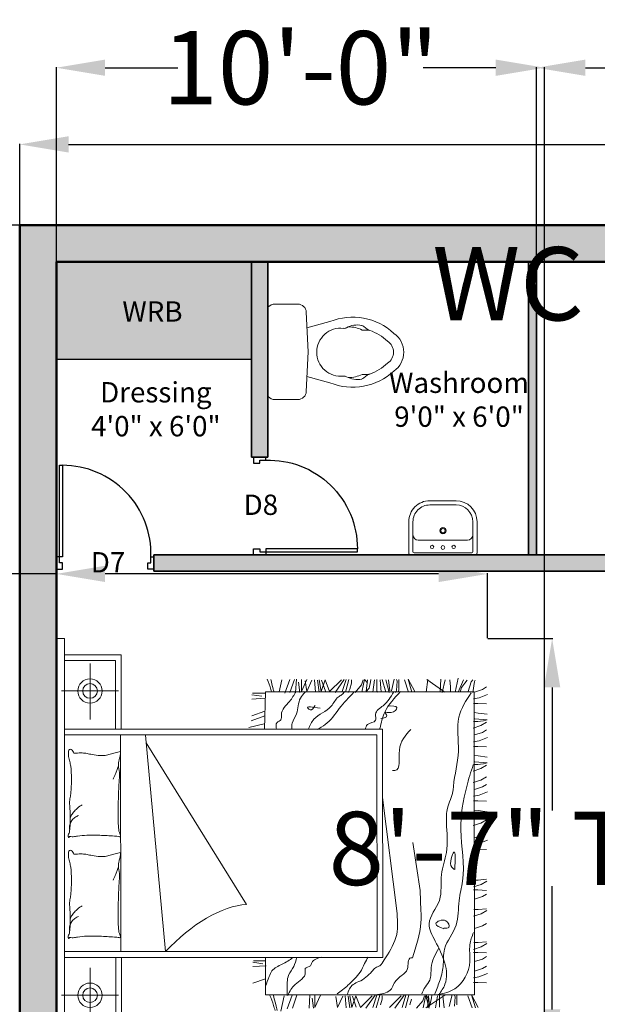
# Model space of a CAD drawing. Units: inches. Extents: x 2796 to 3603, y 978 to 1787.
# Tile 12 of 15: x 3070 to 3212, y 1545 to 1787. Entities that reach past the tile are written whole.
import ezdxf

# ---------------------------------------------------------------- set-up
doc = ezdxf.new("R2010")
doc.units = ezdxf.units.IN
for name, color, linetype, lineweight in [('A-ANNO-DIMS', 7, 'Continuous', 18), ('A-ANNO-TEXT', 7, 'Continuous', 18), ('A-AREA-IDEN', 7, 'Continuous', 18), ('A-DOOR', 6, 'Continuous', 25), ('A-FLOR-CASE', 2, 'Continuous', 25), ('A-FLOR-CASE-PATT', 2, 'Continuous', 13), ('A-FLOR-FIXT', 8, 'Continuous', 18), ('A-WALL-EXTR-PATT', 1, 'Continuous', 13), ('A-WALL-INTR-PATT', 5, 'Continuous', 13), ('Furniture', 2, 'Continuous', 18), ('Inner Wall', 5, 'Continuous', 35), ('Outer Wall', 1, 'Continuous', 50)]:
    doc.layers.add(name, color=color, linetype=linetype, lineweight=lineweight)
doc.styles.get("Standard").update_dxf_attribs({"font": 'arial.ttf'})
doc.dimstyles.get("Standard").update_dxf_attribs({"dimtxt": 18, "dimasz": 12, "dimexe": 0.18, "dimexo": 0.0625, "dimgap": 0.09, "dimtad": 0, "dimtih": 1, "dimtoh": 1, "dimdec": 0, "dimzin": 0, "dimdsep": 46, "dimlunit": 3, "dimtxsty": 'Standard', "dimcen": 0.09, "dimadec": 0, "dimazin": 0, "dimtfac": 1, "dimtdec": 0, "dimtofl": 0, "dimtmove": 0, "dimatfit": 3, "dimfxl": 1, "dimtolj": 1, "dimtzin": 0, "dimarcsym": 0})

# ---------------------------------------------------------------- blocks, each defined once
blk = doc.blocks.new('A$C1308471B')
at = {"ltscale": 20}
for p, q in [((0, 0.4607), (0, 0.0186)), ((0.0354, 0.4793), (0.1495, 0.4793)), ((0.2013, 0.2397), (0.1923, 0.4384)), ((0.1957, 0.3639), (0.3109, 0.3953)), ((0.5021, 0.3528), (0.4724, 0.3528)), ((0.4982, 0.3575), (0.4822, 0.3709)), ((0.2013, 0.2397), (0.1923, 0.0409)), ((0.1959, 0.1193), (0.3109, 0.0879)), ((0.5021, 0.1304), (0.4724, 0.1304)), ((0.4982, 0.1257), (0.4822, 0.1123)), ((0.0354, 0), (0.1495, 0))]:
    blk.add_line(p, q, dxfattribs=at)
for centre, radius, start, end in [((0.006, 0.4607), 0.006, 136.5269, 180), ((0.0354, 0.4328), 0.0465, 90, 136.5269), ((0.1495, 0.4365), 0.0429, 2.5755, 90), ((0.4248, 0.1104), 0.3068, 47.4135, 111.7924), ((0.3654, 0.2416), 0.1206, 83.3523, 180), ((0.3823, 0.3868), 0.0255, 263.3523, 298.5742), ((0.4494, 0.2636), 0.1148, 79.3968, 118.5742), ((0.405, 0.2159), 0.153, 63.502, 90.4522), ((0.4658, 0.3513), 0.0255, 50, 79.3968), ((0.5146, 0.377), 0.0255, 230, 251.3881), ((0.5021, 0.3273), 0.0255, 70.3751, 90), ((0.4248, 0.1104), 0.2558, 46.612, 70.3751), ((0.5654, 0.2416), 0.116, 0, 54.7115), ((0.5654, 0.2416), 0.065, 0, 57.2974), ((0.3654, 0.2416), 0.1206, 180, 276.6477), ((0.5654, 0.2416), 0.065, 302.7026, 0), ((0.5654, 0.2416), 0.116, 305.2885, 0), ((0.4248, 0.3728), 0.2558, 289.6249, 313.388), ((0.4248, 0.3728), 0.3068, 248.2076, 312.5865), ((0.3823, 0.0964), 0.0255, 61.4258, 96.6477), ((0.4494, 0.2196), 0.1148, 241.4258, 280.6032), ((0.405, 0.2673), 0.153, 269.5478, 296.498), ((0.4658, 0.1319), 0.0255, 280.6032, 310), ((0.5146, 0.1062), 0.0255, 108.6119, 130), ((0.5021, 0.1559), 0.0255, 270, 289.6249), ((0.006, 0.0186), 0.006, 180, 223.4731), ((0.0354, 0.0465), 0.0465, 223.4731, 270), ((0.1495, 0.0429), 0.0429, 270, 357.4245)]:
    blk.add_arc(centre, radius, start, end, dxfattribs=at)
blk = doc.blocks.new('A$C57EA129C')
for p, q in [((0, 0.4428), (0, 0.1782)), ((0.016, 0.4589), (0.5631, 0.4589)), ((0.0356, 0.4321), (0.0356, 0.2896)), ((0.0445, 0.441), (0.5346, 0.441)), ((0.5435, 0.4321), (0.5435, 0.2896)), ((0.5791, 0.4428), (0.5791, 0.1782)), ((0.0802, 0.3341), (0.499, 0.3341)), ((0.0356, 0.2896), (0.0356, 0.1782)), ((0.5435, 0.2896), (0.5435, 0.1782)), ((0.1782, 0.0356), (0.4009, 0.0356)), ((0.1782, 0), (0.4009, 0))]:
    blk.add_line(p, q)
for centre, radius in [((0.1982, 0.392), 0.0143), ((0.2896, 0.3965), 0.0156), ((0.3809, 0.392), 0.0143), ((0.2896, 0.2545), 0.0267), ((0.2896, 0.2545), 0.0178)]:
    blk.add_circle(centre, radius)
for centre, radius, start, end in [((0.016, 0.4428), 0.016, 90, 180), ((0.0445, 0.4321), 0.00891, 90, 180), ((0.5346, 0.4321), 0.00891, 0, 90), ((0.5631, 0.4428), 0.016, 0, 90), ((0.0802, 0.2896), 0.0445, 90, 180), ((0.499, 0.2896), 0.0445, 0, 90), ((0.1782, 0.1782), 0.1782, 180, 270), ((0.1782, 0.1782), 0.1426, 180, 270), ((0.4009, 0.1782), 0.1782, 270, 0), ((0.4009, 0.1782), 0.1426, 270, 0)]:
    blk.add_arc(centre, radius, start, end)
blk = doc.blocks.new('A$C2B723114')
for p, q in [((0, 2.9047), (2.8274, 2.9047)), ((0, 2.8487), (0, 2.9047)), ((0.4243, 2.8697), (0.4243, 2.4855)), ((2.4742, 2.8697), (2.4742, 2.4855)), ((2.8274, 2.9047), (2.8274, 2.8487)), ((2.8274, 2.8487), (0, 2.8487)), ((0.1012, 2.4649), (0.1012, 2.849)), ((0.1396, 2.5033), (0.1396, 2.849)), ((0.6794, 0.7051), (0.6794, 2.8509)), ((0.7187, 0.7435), (0.7187, 2.8509)), ((2.1776, 2.8509), (2.1776, 0.7454)), ((2.216, 2.8509), (2.216, 0.707)), ((2.6798, 2.5052), (2.6798, 2.8509)), ((2.7182, 2.4668), (2.7182, 2.8509)), ((0.6087, 2.6776), (0.295, 2.6776)), ((2.6586, 2.6776), (2.2821, 2.6776)), ((1.3789, 2.4999), (1.3598, 2.5761)), ((2.0593, 2.4999), (2.0402, 2.5761)), ((0.6794, 2.4649), (0.1012, 2.4649)), ((0.6766, 2.5033), (0.1396, 2.5033)), ((0.7191, 2.47), (2.1778, 2.4719)), ((1.3858, 2.4723), (1.3789, 2.4999)), ((2.0662, 2.4723), (2.0593, 2.4999)), ((2.2188, 2.5052), (2.6798, 2.5052)), ((2.2188, 2.4668), (2.7182, 2.4668)), ((2.1771, 2.3036), (0.718, 2.1685)), ((1.0365, 1.6233), (2.1246, 2.2989)), ((2.2287, 1.6076), (2.2523, 1.5035)), ((2.2726, 1.593), (2.3061, 1.5007)), ((0.5047, 1.5819), (0.5353, 1.4945)), ((0.6174, 1.5819), (0.6232, 1.4916)), ((0.6467, 1.5819), (0.6369, 1.5137)), ((0.6571, 1.4945), (0.6571, 1.5765)), ((2.3067, 1.5881), (2.3373, 1.5007)), ((2.4194, 1.5881), (2.4251, 1.4979)), ((2.4487, 1.5881), (2.4389, 1.5199)), ((2.4591, 1.5007), (2.4591, 1.5828)), ((0.4269, 0.0884), (0.4269, 1.4945)), ((0.4269, 1.4945), (0.6794, 1.4945)), ((2.4685, 1.4964), (2.216, 1.5022)), ((2.4685, 1.4964), (2.4685, 0.0903)), ((2.4685, 1.4044), (2.5491, 1.3861)), ((0.3172, 1.3923), (0.4213, 1.3687)), ((0.3318, 1.3485), (0.4241, 1.3149)), ((2.4596, 1.3659), (2.552, 1.3324)), ((2.4645, 1.3318), (2.552, 1.3012)), ((0.3367, 1.3143), (0.4241, 1.2838)), ((2.4645, 1.2928), (2.5548, 1.2871)), ((2.4645, 1.2635), (2.5328, 1.2733)), ((0.3367, 1.2016), (0.427, 1.1959)), ((2.4699, 1.2531), (2.552, 1.2163)), ((2.552, 1.2531), (2.4699, 1.2531)), ((2.5435, 1.2276), (2.4699, 1.2163)), ((2.4699, 1.2163), (2.5463, 1.1823)), ((0.3367, 1.1724), (0.405, 1.1821)), ((0.4241, 1.162), (0.3421, 1.162)), ((0.3421, 1.162), (0.4241, 1.1252)), ((2.5491, 1.1654), (2.467, 1.1597)), ((2.5463, 1.1455), (2.467, 1.1342)), ((2.5491, 1.1342), (2.4699, 1.1201)), ((2.4699, 1.1201), (2.5491, 1.0946)), ((2.5491, 1.0946), (2.4699, 1.0635)), ((2.4699, 1.0635), (2.5491, 0.9842)), ((2.5463, 1.1172), (2.4727, 1.0918)), ((0.4157, 1.0206), (0.3421, 1.0093)), ((0.3421, 1.0093), (0.4185, 0.9754)), ((2.4642, 1.0267), (2.552, 0.9644)), ((0.4213, 0.9584), (0.3392, 0.9527)), ((0.4185, 0.9386), (0.3392, 0.9272)), ((2.4642, 0.9389), (2.4869, 0.9276)), ((2.467, 0.9559), (2.552, 0.9333)), ((2.4699, 0.9785), (2.552, 0.9531)), ((0.4213, 0.9272), (0.3421, 0.9131)), ((0.3421, 0.9131), (0.4213, 0.8876)), ((0.4213, 0.8876), (0.3421, 0.8565)), ((0.4185, 0.9103), (0.3449, 0.8848)), ((2.4642, 0.8908), (2.5152, 0.8483)), ((2.4869, 0.9276), (2.5265, 0.9163)), ((2.5265, 0.9163), (2.5491, 0.9163)), ((0.3364, 0.8197), (0.4241, 0.7574)), ((0.3421, 0.8565), (0.4213, 0.7772)), ((2.467, 0.8455), (2.5208, 0.8342)), ((2.4699, 0.8172), (2.4925, 0.7974)), ((2.5491, 0.8087), (2.4699, 0.8172)), ((2.4925, 0.7974), (2.535, 0.7889)), ((2.5152, 0.8483), (2.5491, 0.837)), ((2.5208, 0.8342), (2.552, 0.8285)), ((2.552, 0.8285), (2.5293, 0.8087)), ((0.3392, 0.7489), (0.4241, 0.7263)), ((0.3421, 0.7716), (0.4241, 0.7461)), ((2.1776, 0.7454), (0.7187, 0.7435)), ((2.5491, 0.7606), (2.467, 0.7719)), ((2.4727, 0.7464), (2.467, 0.7408)), ((2.552, 0.7464), (2.4727, 0.7464)), ((2.535, 0.7889), (2.552, 0.7861)), ((0.359, 0.7206), (0.3987, 0.7093)), ((0.3987, 0.7093), (0.4213, 0.7093)), ((2.216, 0.707), (0.6794, 0.7051)), ((0.9938, 0.6115), (1.7555, 0.7064)), ((2.5491, 0.6842), (2.4642, 0.6615)), ((2.467, 0.7153), (2.5491, 0.7238)), ((2.552, 0.7096), (2.467, 0.6842)), ((2.5491, 0.6672), (2.4755, 0.6587)), ((0.3364, 0.6233), (0.4241, 0.561)), ((0.3421, 0.6601), (0.4213, 0.5808)), ((2.4642, 0.6191), (2.4784, 0.6134)), ((2.467, 0.5993), (2.4869, 0.5964)), ((2.4755, 0.6474), (2.5548, 0.6276)), ((2.4784, 0.6134), (2.5406, 0.6077)), ((2.5406, 0.6077), (2.552, 0.6134)), ((0.3392, 0.5525), (0.4241, 0.5299)), ((0.3421, 0.5752), (0.4241, 0.5497)), ((2.467, 0.5313), (2.5491, 0.5596)), ((2.467, 0.5087), (2.5548, 0.5342)), ((2.5548, 0.5342), (2.4699, 0.4889)), ((2.4869, 0.5964), (2.552, 0.5964)), ((0.3364, 0.4785), (0.3874, 0.436)), ((0.359, 0.5242), (0.3987, 0.5129)), ((1.4523, 0.5021), (1.1305, 0.4537)), ((0.4213, 0.415), (0.3364, 0.3923)), ((0.3392, 0.4332), (0.393, 0.4219)), ((0.4241, 0.2868), (0.3392, 0.415)), ((0.3421, 0.4049), (0.3647, 0.3851)), ((0.4213, 0.3964), (0.3421, 0.4049)), ((0.3874, 0.436), (0.4213, 0.4247)), ((0.393, 0.4219), (0.4241, 0.4162)), ((0.4241, 0.4162), (0.4015, 0.3964)), ((1.1305, 0.4537), (0.9938, 0.448)), ((2.467, 0.4133), (2.552, 0.4019)), ((2.467, 0.2879), (2.552, 0.4076)), ((0.4213, 0.3377), (0.3392, 0.3491)), ((0.4213, 0.398), (0.3477, 0.3895)), ((0.3647, 0.3851), (0.4072, 0.3766)), ((0.4072, 0.3766), (0.4241, 0.3738)), ((0.3392, 0.2925), (0.4213, 0.3009)), ((0.4241, 0.3236), (0.3449, 0.3236)), ((2.4642, 0.3049), (2.5491, 0.2851)), ((2.467, 0.319), (2.5548, 0.3134)), ((0.3477, 0.2571), (0.427, 0.2373)), ((0.3506, 0.2231), (0.4128, 0.2175)), ((0.359, 0.2061), (0.4241, 0.2061)), ((0.4128, 0.2175), (0.4241, 0.2231)), ((2.467, 0.2179), (2.5605, 0.1981)), ((2.4699, 0.2491), (2.501, 0.2491)), ((2.501, 0.2491), (2.5491, 0.2547)), ((2.467, 0.1981), (2.5491, 0.1613)), ((2.467, 0.184), (2.4982, 0.1755)), ((2.4982, 0.1755), (2.5463, 0.1359)), ((0.3392, 0.1042), (0.4213, 0.1325)), ((0.3392, 0.0815), (0.427, 0.107)), ((0.427, 0.107), (0.3421, 0.0617)), ((2.4685, 0.0903), (0.4269, 0.0884)), ((0.5106, 0.094), (0.5106, 0.0657)), ((0.5417, 0.094), (0.5474, 0.0572)), ((0.587, 0.0884), (0.604, 0.0346)), ((0.6512, 0.0884), (0.6682, 0.0346)), ((0.713, 0.094), (0.713, 0.0657)), ((0.7334, 0.0943), (0.7503, 0.0434)), ((0.7786, 0.0915), (0.7786, 0.0632)), ((0.8739, 0.0884), (0.8908, 0.0346)), ((0.956, 0.0943), (0.973, 0.0434)), ((1.0013, 0.0915), (1.0013, 0.0632)), ((1.072, 0.0884), (1.089, 0.0346)), ((1.1338, 0.094), (1.1338, 0.0657)), ((1.1542, 0.0943), (1.1712, 0.0434)), ((1.1995, 0.0915), (1.1995, 0.0632)), ((1.4088, 0.094), (1.4088, 0.0657)), ((1.44, 0.094), (1.4456, 0.0572)), ((1.4853, 0.0884), (1.5023, 0.0346)), ((1.5674, 0.0962), (1.5844, 0.0453)), ((1.6127, 0.0934), (1.6127, 0.0651)), ((1.6297, 0.0849), (1.624, 0.0028)), ((1.6721, 0.0877), (1.6693, 0.0623)), ((1.7344, 0.0934), (1.7344, 0.0651)), ((1.7655, 0.0934), (1.7712, 0.0566)), ((1.8108, 0.0877), (1.8278, 0.034)), ((1.8568, 0.0962), (1.8738, 0.0453)), ((1.9342, 0.0962), (1.9512, 0.0453)), ((1.9795, 0.0934), (1.9795, 0.0651)), ((1.9965, 0.0849), (1.9908, 0.0028)), ((2.039, 0.0877), (2.0361, 0.0623)), ((2.1012, 0.0934), (2.1012, 0.0651)), ((2.1324, 0.0934), (2.138, 0.0566)), ((2.1777, 0.0877), (2.1946, 0.034)), ((2.2236, 0.0962), (2.2406, 0.0453)), ((2.2689, 0.0934), (2.2689, 0.0651)), ((2.2859, 0.0849), (2.2802, 0.0028)), ((2.3284, 0.0877), (2.3255, 0.0623)), ((2.3906, 0.0934), (2.3906, 0.0651)), ((2.4218, 0.0934), (2.4274, 0.0566)), ((2.4642, 0.0991), (2.5378, 0.0877)), ((2.467, 0.0877), (2.484, 0.034)), ((2.4699, 0.1302), (2.535, 0.1104)), ((2.535, 0.1104), (2.5491, 0.0991)), ((2.5378, 0.0877), (2.5463, 0.0821)), ((0.5106, 0.0657), (0.5077, 0.0063)), ((0.5474, 0.0572), (0.57, 0.0006)), ((0.604, 0.0346), (0.621, 0.0063)), ((0.6682, 0.0346), (0.6851, 0.0063)), ((0.713, 0.0657), (0.7101, 0.0063)), ((0.7503, 0.0434), (0.773, 0.0037)), ((0.7786, 0.0632), (0.7843, 0.0066)), ((0.8908, 0.0346), (0.9078, 0.0063)), ((0.973, 0.0434), (0.9957, 0.0037)), ((1.0013, 0.0632), (1.007, 0.0066)), ((1.089, 0.0346), (1.106, 0.0063)), ((1.1338, 0.0657), (1.131, 0.0063)), ((1.1712, 0.0434), (1.1939, 0.0037)), ((1.1995, 0.0632), (1.2052, 0.0066)), ((1.4088, 0.0657), (1.406, 0.0063)), ((1.4456, 0.0572), (1.4683, 0.0006)), ((1.5023, 0.0346), (1.5192, 0.0082)), ((1.5844, 0.0453), (1.607, 0.0057)), ((1.6127, 0.0651), (1.6184, 0.0085)), ((1.6693, 0.0623), (1.6608, 0.0028)), ((1.7344, 0.0651), (1.7316, 0.0057)), ((1.7712, 0.0566), (1.7938, 0)), ((1.8278, 0.034), (1.8448, 0.0057)), ((1.8738, 0.0453), (1.8964, 0.0057)), ((1.9512, 0.0453), (1.9739, 0.0057)), ((1.9795, 0.0651), (1.9852, 0.0085)), ((2.0361, 0.0623), (2.0276, 0.0028)), ((2.1012, 0.0651), (2.0984, 0.0057)), ((2.138, 0.0566), (2.1607, 0)), ((2.1946, 0.034), (2.2116, 0.0057)), ((2.2406, 0.0453), (2.2632, 0.0057)), ((2.2689, 0.0651), (2.2746, 0.0085)), ((2.3255, 0.0623), (2.317, 0.0028)), ((2.3906, 0.0651), (2.3878, 0.0057)), ((2.4274, 0.0566), (2.4501, 0)), ((2.484, 0.034), (2.501, 0.0057))]:
    blk.add_line(p, q)
for centre, radius in [((0.4243, 2.6776), 0.0821), ((0.4243, 2.6776), 0.0493), ((2.4742, 2.6776), 0.0821), ((2.4742, 2.6776), 0.0493)]:
    blk.add_circle(centre, radius)
for centre, radius, start, end in [((0.8078, 2.821), 0.00214, 160.43603, 281.89306), ((0.8088, 2.8207), 0.00315, 111.7883, 160.43603), ((0.8162, 2.8021), 0.0232, 94.30254, 111.7883), ((0.8091, 2.8151), 0.00394, 21.9904, 101.89306), ((0.8409, 2.7949), 0.0302, 158.57902, 188.13348), ((1.0356, 2.8227), 0.2268, 188.13348, 192.10946), ((0.7994, 2.8112), 0.0144, 338.57902, 21.9904), ((0.8165, 2.7987), 0.0266, 59.34875, 94.30254), ((0.8554, 2.8643), 0.0497, 239.34875, 264.74081), ((0.9202, 3.5684), 0.7568, 264.74081, 268.09211), ((0.8679, 2.7254), 0.0915, 74.06476, 94.21588), ((0.8679, 2.7254), 0.0915, 53.91364, 74.06476), ((0.9409, 4.189), 1.3777, 268.09211, 270.57574), ((0.8679, 2.7254), 0.0915, 36.17665, 53.91364), ((0.86, 2.6097), 0.2158, 62.76041, 69.13972), ((0.9466, 3.6164), 0.8051, 270.57574, 274.80185), ((0.9263, 2.7386), 0.0708, 51.61143, 62.76041), ((0.7461, 2.511), 0.3611, 46.18849, 51.61143), ((1.0364, 2.548), 0.2671, 87.46141, 94.80185), ((1.042, 2.6745), 0.1405, 79.81012, 87.46141), ((1.1532, 3.2931), 0.488, 259.81012, 263.9133), ((1.204, 3.7695), 0.9671, 263.9133, 270), ((1.204, 3.4318), 0.6294, 270, 277.54685), ((1.2573, 3.0292), 0.2233, 277.54685, 285.74398), ((1.3941, 2.5438), 0.281, 98.43719, 105.74398), ((1.3747, 2.6748), 0.1486, 90, 98.43719), ((1.3713, 2.8186), 0.0315, 274.40021, 333.41948), ((0.923, 2.7382), 0.4535, 0, 6.23236), ((1.3747, 2.74), 0.0833, 78.72762, 90), ((1.3886, 2.8099), 0.0121, 333.41948, 78.72762), ((1.4882, 2.821), 0.00214, 160.43603, 281.89306), ((1.4892, 2.8207), 0.00315, 111.7883, 160.43603), ((1.4966, 2.8021), 0.0232, 94.30254, 111.7883), ((1.4895, 2.8151), 0.00394, 21.9904, 101.89306), ((1.5213, 2.7949), 0.0302, 158.57902, 188.13348), ((1.716, 2.8227), 0.2268, 188.13348, 192.10946), ((1.4798, 2.8112), 0.0144, 338.57902, 21.9904), ((1.4969, 2.7987), 0.0266, 59.34875, 94.30254), ((1.5358, 2.8643), 0.0497, 239.34875, 264.74081), ((1.6006, 3.5684), 0.7568, 264.74081, 268.09211), ((1.5483, 2.7254), 0.0915, 74.06476, 94.21588), ((1.5483, 2.7254), 0.0915, 53.91364, 74.06476), ((1.6213, 4.189), 1.3777, 268.09211, 270.57574), ((1.5483, 2.7254), 0.0915, 36.17665, 53.91364), ((1.5404, 2.6097), 0.2158, 62.76041, 69.13972), ((1.627, 3.6164), 0.8051, 270.57574, 274.80185), ((1.6067, 2.7386), 0.0708, 51.61143, 62.76041), ((1.4265, 2.511), 0.3611, 46.18849, 51.61143), ((1.7168, 2.548), 0.2671, 87.46141, 94.80185), ((1.7224, 2.6745), 0.1405, 79.81012, 87.46141), ((1.8336, 3.2931), 0.488, 259.81012, 263.9133), ((1.8844, 3.7695), 0.9671, 263.9133, 270), ((1.8844, 3.4318), 0.6294, 270, 277.54685), ((1.9377, 3.0292), 0.2233, 277.54685, 285.74398), ((2.0745, 2.5438), 0.281, 98.43719, 105.74398), ((2.0551, 2.6748), 0.1486, 90, 98.43719), ((2.0517, 2.8186), 0.0315, 274.40021, 333.41948), ((1.6034, 2.7382), 0.4535, 0, 6.23236), ((2.0551, 2.74), 0.0833, 78.72762, 90), ((2.069, 2.8099), 0.0121, 333.41948, 78.72762), ((0.635, 2.7368), 0.1829, 7.6809, 12.10946), ((-0.0181, 2.6487), 0.8418, 3.36875, 7.6809), ((0.8679, 2.7254), 0.0915, 18.43965, 36.17665), ((0.8523, 2.6218), 0.2076, 39.03494, 46.18849), ((0.9783, 2.7239), 0.0455, 28.31676, 39.03494), ((0.8558, 2.6579), 0.1846, 23.00277, 28.31676), ((1.1884, 2.7382), 0.1881, 350.31563, 0), ((1.3154, 2.7368), 0.1829, 7.6809, 12.10946), ((0.6623, 2.6487), 0.8418, 3.36875, 7.6809), ((1.5483, 2.7254), 0.0915, 18.43965, 36.17665), ((1.5327, 2.6218), 0.2076, 39.03494, 46.18849), ((1.6587, 2.7239), 0.0455, 28.31676, 39.03494), ((1.5362, 2.6579), 0.1846, 23.00277, 28.31676), ((1.8688, 2.7382), 0.1881, 350.31563, 0), ((0.1976, 2.6614), 0.6258, 358.36691, 3.36875), ((1.6528, 2.6098), 0.2924, 167.80162, 171.99495), ((0.5722, 2.8434), 0.8132, 347.80162, 350.31563), ((0.878, 2.6614), 0.6258, 358.36691, 3.36875), ((2.3332, 2.6098), 0.2924, 167.80162, 171.99495), ((1.2526, 2.8434), 0.8132, 347.80162, 350.31563), ((-11.7321, 3.2823), 12.5718, 356.49514, 356.94504), ((-0.4351, 2.6794), 1.2587, 356.94504, 358.36691), ((1.9648, 2.5659), 0.6074, 171.99495, 177.33512), ((1.4204, 2.5912), 0.0624, 177.33512, 194.04519), ((-11.0517, 3.2823), 12.5718, 356.49514, 356.94504), ((0.2453, 2.6794), 1.2587, 356.94504, 358.36691), ((2.6452, 2.5659), 0.6074, 171.99495, 177.33512), ((2.1008, 2.5912), 0.0624, 177.33512, 194.04519), ((0.8298, 2.4774), 0.0178, 170.00164, 196.69777), ((0.5206, 2.5319), 0.2961, 350.00164, 356.49514), ((0.8139, 2.4726), 0.00122, 196.69777, 277.12039), ((0.8041, 2.5514), 0.0807, 277.12039, 286.22115), ((0.8068, 2.5419), 0.0707, 286.22115, 297.28412), ((0.8584, 2.4419), 0.0418, 102.86904, 117.28412), ((0.879, 2.3515), 0.1345, 93.57397, 102.86904), ((0.9376, 1.4146), 1.0732, 90.28654, 93.57397), ((0.9586, -2.7845), 5.2724, 89.02962, 90.28654), ((0.9954, -0.6123), 3.0999, 87.39037, 89.02962), ((1.0854, 1.364), 1.1216, 85.38242, 87.39037), ((1.28, 3.7729), 1.2952, 265.38242, 267.25094), ((1.4917, 3.1364), 0.681, 244.68893, 246.51559), ((1.228, 2.691), 0.2121, 267.25094, 281.55856), ((1.4917, 3.1364), 0.681, 246.51559, 248.34226), ((1.4917, 3.1364), 0.681, 248.34226, 250.57202), ((1.4917, 3.1364), 0.681, 250.57202, 252.80178), ((1.2975, 2.3514), 0.1345, 83.56595, 101.55856), ((1.3002, 2.3754), 0.1104, 72.61359, 83.56595), ((1.3965, 2.6828), 0.2118, 252.61359, 260.5159), ((1.4027, 2.7202), 0.2496, 260.5159, 265.91706), ((1.385, 2.4721), 0.000845, 265.91706, 14.04494), ((1.5102, 2.4774), 0.0178, 170.00164, 196.69777), ((1.201, 2.5319), 0.2961, 350.00164, 356.49514), ((1.4943, 2.4726), 0.00122, 196.69777, 277.12039), ((1.4845, 2.5514), 0.0807, 277.12039, 286.22115), ((1.4872, 2.5419), 0.0707, 286.22115, 297.28412), ((1.5388, 2.4419), 0.0418, 102.86904, 117.28412), ((1.5594, 2.3515), 0.1345, 93.57397, 102.86904), ((1.618, 1.4146), 1.0732, 90.28654, 93.57397), ((1.639, -2.7845), 5.2724, 89.02962, 90.28654), ((1.6758, -0.6123), 3.0999, 87.39037, 89.02962), ((1.7658, 1.364), 1.1216, 85.38242, 87.39037), ((1.9604, 3.7729), 1.2952, 265.38242, 267.25094), ((2.1721, 3.1364), 0.681, 244.68893, 246.51559), ((1.9084, 2.691), 0.2121, 267.25094, 281.55856), ((2.1721, 3.1364), 0.681, 246.51559, 248.34226), ((2.1721, 3.1364), 0.681, 248.34226, 250.57202), ((2.1721, 3.1364), 0.681, 250.57202, 252.80178), ((1.9779, 2.3514), 0.1345, 83.56595, 101.55856), ((1.9806, 2.3754), 0.1104, 72.61359, 83.56595), ((2.0769, 2.6828), 0.2118, 252.61359, 260.5159), ((2.0831, 2.7202), 0.2496, 260.5159, 265.91706), ((2.0654, 2.4721), 0.000845, 265.91706, 14.04494)]:
    blk.add_arc(centre, radius, start, end)
blk.add_ellipse((0.4962, 1.9132), major_axis=(0.4887, -0.4605), ratio=0.503305, start_param=0.491272, end_param=1.591113)
for points, knots in [([(0.427, 1.4678), (0.4036, 1.4582), (0.3693, 1.4441), (0.3335, 1.4344), (0.3221, 1.4313)], [0, 0, 0, 0, 98.452083, 144.639601, 144.639601, 144.639601, 144.639601]), ([(0.6768, 1.3104), (0.6615, 1.3339), (0.6315, 1.3797), (0.604, 1.4501), (0.5417, 1.4748), (0.5064, 1.4871), (0.4848, 1.4945)], [0, 0, 0, 0, 110.980521, 216.571322, 273.316778, 363.252298, 363.252298, 363.252298, 363.252298]), ([(2.5548, 1.4853), (2.5314, 1.4757), (2.5031, 1.4641), (2.4737, 1.4555), (2.4685, 1.454)], [0, 0, 0, 0, 98.452083, 119.481049, 119.481049, 119.481049, 119.481049]), ([(2.552, 1.4598), (2.5309, 1.4545), (2.5031, 1.4475), (2.4753, 1.4406), (2.4685, 1.4389)], [0, 0, 0, 0, 84.638756, 111.94623, 111.94623, 111.94623, 111.94623]), ([(0.4241, 1.4423), (0.4031, 1.437), (0.3691, 1.4284), (0.3351, 1.4199), (0.3221, 1.4167)], [0, 0, 0, 0, 84.638756, 136.955563, 136.955563, 136.955563, 136.955563]), ([(2.2145, 1.4211), (2.233, 1.4246), (2.2636, 1.4303), (2.2761, 1.3837), (2.3429, 1.3967), (2.3949, 1.3342), (2.4474, 1.3031), (2.4698, 1.2898)], [0, 0, 0, 0, 61.886907, 102.717887, 145.699352, 284.082577, 386.765171, 386.765171, 386.765171, 386.765171]), ([(0.6768, 1.286), (0.6567, 1.2911), (0.6145, 1.3017), (0.5543, 1.3533), (0.4816, 1.349), (0.4362, 1.3493), (0.4233, 1.3493)], [0, 0, 0, 0, 80.250278, 168.388677, 295.908361, 346.663112, 346.663112, 346.663112, 346.663112]), ([(0.4233, 1.3445), (0.4367, 1.3385), (0.464, 1.3264), (0.5129, 1.2848), (0.5456, 1.2161), (0.6131, 1.2349), (0.6142, 1.1913), (0.6642, 1.1806), (0.674, 1.144), (0.6817, 1.1154)], [0, 0, 0, 0, 56.745495, 115.23739, 254.956954, 286.678662, 337.828324, 366.201072, 468.500395, 468.500395, 468.500395, 468.500395]), ([(2.2145, 1.319), (2.2295, 1.319), (2.2678, 1.3192), (2.3288, 1.2705), (2.4143, 1.279), (2.4535, 1.2403), (2.4662, 1.2278)], [0, 0, 0, 0, 57.155505, 146.33427, 287.936209, 355.396728, 355.396728, 355.396728, 355.396728]), ([(2.2182, 1.2059), (2.2419, 1.1958), (2.3116, 1.1659), (2.342, 1.0552), (2.4266, 1.0223), (2.4474, 0.9811), (2.462, 0.9684), (2.4698, 0.9616)], [0, 0, 0, 0, 97.73655, 287.59661, 389.176293, 423.403759, 463.679181, 463.679181, 463.679181, 463.679181]), ([(2.3573, 1.127), (2.3656, 1.1759), (2.3758, 1.2352), (2.3371, 1.1853), (2.3602, 1.1713), (2.3768, 1.1612)], [0, 0, 0, 0, 107.853607, 130.728419, 189.220329, 189.220329, 189.220329, 189.220329]), ([(2.2145, 1.1476), (2.2246, 1.1286), (2.2575, 1.0666), (2.3612, 1.0009), (2.431, 0.9336), (2.4662, 0.8996)], [0, 0, 0, 0, 83.02987, 271.460712, 463.033803, 463.033803, 463.033803, 463.033803]), ([(0.6817, 0.8034), (0.6673, 0.8119), (0.6341, 0.8315), (0.5785, 0.8518), (0.5349, 0.8973), (0.4828, 0.9461), (0.4518, 0.9879), (0.4331, 1.013)], [0, 0, 0, 0, 65.318952, 150.437229, 226.833166, 307.58338, 429.454095, 429.454095, 429.454095, 429.454095]), ([(0.4282, 0.9448), (0.4547, 0.9353), (0.496, 0.9206), (0.5223, 0.8436), (0.5628, 0.7946), (0.6113, 0.7575), (0.6214, 0.7173), (0.6539, 0.7022), (0.672, 0.6897), (0.6768, 0.6864)], [0, 0, 0, 0, 102.299436, 159.044876, 303.717955, 348.579152, 391.138254, 454.581655, 477.456496, 477.456496, 477.456496, 477.456496]), ([(2.2145, 0.823), (2.227, 0.8201), (2.261, 0.8121), (2.261, 0.7401), (2.3352, 0.7659), (2.379, 0.6836), (2.4336, 0.6521), (2.4662, 0.6334)], [0, 0, 0, 0, 46.747668, 127.438174, 179.649794, 280.561838, 429.605131, 429.605131, 429.605131, 429.605131]), ([(0.4282, 0.74), (0.4347, 0.7029), (0.444, 0.6496), (0.5194, 0.6274), (0.555, 0.5807), (0.5975, 0.5243), (0.6789, 0.5415), (0.677, 0.5095), (0.6768, 0.5061)], [0, 0, 0, 0, 130.791737, 187.537266, 286.231946, 353.673191, 460.023761, 472.712403, 472.712403, 472.712403, 472.712403]), ([(0.6768, 0.6864), (0.7275, 0.655), (0.8251, 0.5944), (0.9391, 0.606), (0.9938, 0.6115)], [0, 0, 0, 0, 225.995823, 434.686543, 434.686543, 434.686543, 434.686543]), ([(2.2218, 0.7246), (2.2595, 0.716), (2.3548, 0.6945), (2.4265, 0.6268), (2.4698, 0.586)], [0, 0, 0, 0, 148.665024, 375.555892, 375.555892, 375.555892, 375.555892]), ([(2.3719, 0.6737), (2.3738, 0.6431), (2.3772, 0.5878), (2.3146, 0.6382), (2.3401, 0.7015), (2.2971, 0.6649), (2.2923, 0.6965), (2.289, 0.7176)], [0, 0, 0, 0, 83.446591, 150.887818, 201.642461, 230.015204, 286.760644, 286.760644, 286.760644, 286.760644]), ([(2.2145, 0.5167), (2.1764, 0.5522), (2.1051, 0.6184), (1.9357, 0.5803), (1.9385, 0.6342), (1.9388, 0.6395)], [0, 0, 0, 0, 208.073343, 389.01094, 409.01094, 409.01094, 409.01094, 409.01094]), ([(0.6768, 0.5061), (0.7554, 0.4794), (0.8591, 0.4442), (0.9675, 0.4473), (0.9938, 0.448)], [0, 0, 0, 0, 319.374611, 421.61723, 421.61723, 421.61723, 421.61723]), ([(0.4331, 0.4427), (0.4498, 0.4356), (0.4827, 0.4216), (0.5314, 0.3759), (0.632, 0.3884), (0.6996, 0.3513), (0.7423, 0.3278)], [0, 0, 0, 0, 70.931849, 139.556414, 248.154027, 434.709995, 434.709995, 434.709995, 434.709995]), ([(2.4625, 0.1088), (2.4095, 0.1438), (2.2904, 0.2226), (2.0623, 0.1771), (1.9006, 0.2246), (1.7699, 0.2337), (1.6941, 0.2766), (1.5528, 0.2786), (1.4005, 0.2587), (1.2324, 0.3267), (1.059, 0.2939), (0.9218, 0.426), (0.7359, 0.3204), (0.5586, 0.2391), (0.4502, 0.3116), (0.427, 0.3272)], [0, 0, 0, 0, 239.874704, 538.942419, 850.40885, 893.390315, 1047.998294, 1176.505142, 1437.500972, 1637.333004, 1864.324391, 2089.058767, 2248.736533, 2637.953392, 2744.252142, 2744.252142, 2744.252142, 2744.252142]), ([(1.9771, 0.0962), (1.9286, 0.1117), (1.7864, 0.157), (1.5223, 0.1992), (1.2611, 0.141), (1.0527, 0.2023), (0.8859, 0.1885), (0.76, 0.3042), (0.6211, 0.292), (0.5187, 0.3203), (0.4572, 0.3456), (0.4282, 0.3575)], [0, 0, 0, 0, 198.710624, 582.73994, 1031.873213, 1206.082894, 1423.278209, 1655.952104, 1808.744089, 1945.69963, 2068.229211, 2068.229211, 2068.229211, 2068.229211]), ([(0.8474, 0.0943), (0.82, 0.1047), (0.757, 0.1287), (0.6201, 0.1029), (0.4623, 0.1837), (0.4372, 0.2936), (0.4282, 0.3331)], [0, 0, 0, 0, 112.422038, 258.341957, 533.791494, 688.286079, 688.286079, 688.286079, 688.286079]), ([(0.8718, 0.2941), (0.8821, 0.3221), (0.9041, 0.3814), (0.9523, 0.2773), (0.8733, 0.2454), (0.8757, 0.2798), (0.8766, 0.2941)], [0, 0, 0, 0, 82.720021, 175.094899, 237.579423, 282.440623, 282.440623, 282.440623, 282.440623]), ([(1.2715, 0.221), (1.3344, 0.2172), (1.4529, 0.21), (1.2971, 0.2665), (1.2756, 0.2284), (1.2715, 0.221)], [0, 0, 0, 0, 150.888188, 283.977876, 315.699589, 315.699589, 315.699589, 315.699589])]:
    blk.add_open_spline(points, degree=3, knots=knots)
blk = doc.blocks.new('*D12')
at = {"layer": 'A-ANNO-DIMS', "color": 0, "lineweight": -2, "transparency": 16777216}
for p, q in [((3070.18, 1736.68), (3041.33, 1736.68)), ((3041.51, 1724.68), (3041.51, 1391.96)), ((3041.51, 1040.68), (3041.51, 1373.4)), ((3070.18, 1028.68), (3041.33, 1028.68))]:
    blk.add_line(p, q, dxfattribs=at)
at = {"layer": 'A-ANNO-DIMS', "color": 0, "transparency": 16777216}
for points in [[(3039.51, 1724.68), (3043.51, 1724.68), (3041.51, 1736.68)], [(3039.51, 1040.68), (3043.51, 1040.68), (3041.51, 1028.68)]]:
    blk.add_solid(points, dxfattribs=at)
at = {"layer": 'Defpoints', "color": 0, "transparency": 16777216}
for p in [(3041.51, 1736.68), (3070.25, 1736.68), (3070.25, 1028.68)]:
    blk.add_point(p, dxfattribs=at)
at = {"layer": 'A-ANNO-DIMS', "color": 0, "transparency": 16777216, "insert": (3041.51, 1382.68), "char_height": 18, "attachment_point": 5}
blk.add_mtext("\\A1;59'", dxfattribs=at)
blk = doc.blocks.new('*D13')
at = {"layer": 'A-ANNO-DIMS', "color": 0, "lineweight": -2, "transparency": 16777216}
for p, q in [((3070.25, 1736.74), (3070.25, 1756.72)), ((3424.25, 1736.74), (3424.25, 1756.72)), ((3082.25, 1756.54), (3216.09, 1756.54)), ((3412.25, 1756.54), (3278.41, 1756.54))]:
    blk.add_line(p, q, dxfattribs=at)
at = {"layer": 'A-ANNO-DIMS', "color": 0, "transparency": 16777216}
for points in [[(3082.25, 1758.54), (3082.25, 1754.54), (3070.25, 1756.54)], [(3412.25, 1758.54), (3412.25, 1754.54), (3424.25, 1756.54)]]:
    blk.add_solid(points, dxfattribs=at)
at = {"layer": 'Defpoints', "color": 0, "transparency": 16777216}
for p in [(3424.25, 1756.54), (3070.25, 1736.68), (3424.25, 1736.68)]:
    blk.add_point(p, dxfattribs=at)
at = {"layer": 'A-ANNO-DIMS', "color": 0, "transparency": 16777216, "insert": (3247.25, 1756.54), "char_height": 18, "attachment_point": 5}
blk.add_mtext('\\A1;29\'-6"', dxfattribs=at)
blk = doc.blocks.new('DOOR-SWING-24IN')
for points in [[(-0.75, -0.7375), (-0.75, 21.7625), (0, 21.7625), (0, -0.7375)], [(-1.5, -3.7375), (0, -3.7375), (0, -2.2375), (-0.75, -2.2375), (-0.75, -0.7375), (-1.5, -0.7375)], [(22.5, -3.7375), (21, -3.7375), (21, -2.2375), (21.75, -2.2375), (21.75, -0.7375), (22.5, -0.7375)]]:
    blk.add_lwpolyline(points, close=True)
blk.add_arc((0, 0), 21.7625, 358.057956, 90)
blk = doc.blocks.new('*D24')
at = {"layer": 'A-ANNO-DIMS', "color": 0, "lineweight": -2, "transparency": 16777216}
for p, q in [((3381.89, 1722.3), (3369.89, 1722.3)), ((3381.89, 1717.36), (3381.89, 1722.48)), ((3403.25, 1722.3), (3393.89, 1722.3)), ((3415.25, 1717.36), (3415.25, 1722.48))]:
    blk.add_line(p, q, dxfattribs=at)
at = {"layer": 'A-ANNO-DIMS', "color": 0, "transparency": 16777216}
for points in [[(3393.89, 1724.3), (3393.89, 1720.3), (3381.89, 1722.3)], [(3403.25, 1724.3), (3403.25, 1720.3), (3415.25, 1722.3)]]:
    blk.add_solid(points, dxfattribs=at)
at = {"layer": 'Defpoints', "color": 0, "transparency": 16777216}
for p in [(3381.89, 1722.3), (3381.89, 1717.3), (3415.25, 1717.3)]:
    blk.add_point(p, dxfattribs=at)
at = {"layer": 'A-ANNO-DIMS', "color": 0, "transparency": 16777216, "insert": (3269.16, 1722.3), "char_height": 18, "attachment_point": 5}
blk.add_mtext('\\A1;WC 2\'-9 1/2" TYP.', dxfattribs=at)
blk = doc.blocks.new('*D26')
at = {"layer": 'A-ANNO-DIMS', "color": 0, "lineweight": -2, "transparency": 16777216}
for p, q in [((3079.25, 1650.99), (3067.25, 1650.99)), ((3079.25, 1635.16), (3079.25, 1651.17)), ((3173.2, 1650.99), (3091.25, 1650.99)), ((3185.2, 1635.16), (3185.2, 1651.17))]:
    blk.add_line(p, q, dxfattribs=at)
at = {"layer": 'A-ANNO-DIMS', "color": 0, "transparency": 16777216}
for points in [[(3091.25, 1652.99), (3091.25, 1648.99), (3079.25, 1650.99)], [(3173.2, 1652.99), (3173.2, 1648.99), (3185.2, 1650.99)]]:
    blk.add_solid(points, dxfattribs=at)
at = {"layer": 'Defpoints', "color": 0, "transparency": 16777216}
for p in [(3079.25, 1650.99), (3079.25, 1635.1), (3185.2, 1635.1)]:
    blk.add_point(p, dxfattribs=at)
at = {"layer": 'A-ANNO-DIMS', "color": 0, "transparency": 16777216, "insert": (2926.76, 1650.99), "char_height": 18, "attachment_point": 5}
blk.add_mtext('\\A1;BED GROUP 8\'-10" TYP.', dxfattribs=at)
blk = doc.blocks.new('*D27')
at = {"layer": 'A-ANNO-DIMS', "color": 0, "lineweight": -2, "transparency": 16777216}
for p, q in [((3185.26, 1635.1), (3201.27, 1635.1)), ((3201.09, 1623.1), (3201.09, 1592.81)), ((3201.09, 1543.97), (3201.09, 1574.25)), ((3185.26, 1531.97), (3201.27, 1531.97))]:
    blk.add_line(p, q, dxfattribs=at)
at = {"layer": 'A-ANNO-DIMS', "color": 0, "transparency": 16777216}
for points in [[(3199.09, 1623.1), (3203.09, 1623.1), (3201.09, 1635.1)], [(3199.09, 1543.97), (3203.09, 1543.97), (3201.09, 1531.97)]]:
    blk.add_solid(points, dxfattribs=at)
at = {"layer": 'Defpoints', "color": 0, "transparency": 16777216}
for p in [(3185.2, 1635.1), (3201.09, 1635.1), (3185.2, 1531.97)]:
    blk.add_point(p, dxfattribs=at)
at = {"layer": 'A-ANNO-DIMS', "color": 0, "transparency": 16777216, "insert": (3201.09, 1583.53), "char_height": 18, "attachment_point": 5}
blk.add_mtext('\\A1;8\'-7" TYP.', dxfattribs=at)
blk = doc.blocks.new('*D40')
at = {"layer": 'A-ANNO-DIMS', "color": 0, "lineweight": -2, "transparency": 16777216}
for p, q in [((3079.25, 1455.74), (3079.25, 1775.56)), ((3091.25, 1775.38), (3109.09, 1775.38)), ((3187.25, 1775.38), (3169.41, 1775.38)), ((3199.25, 1455.74), (3199.25, 1775.56))]:
    blk.add_line(p, q, dxfattribs=at)
at = {"layer": 'A-ANNO-DIMS', "color": 0, "transparency": 16777216}
for points in [[(3091.25, 1777.38), (3091.25, 1773.38), (3079.25, 1775.38)], [(3187.25, 1777.38), (3187.25, 1773.38), (3199.25, 1775.38)]]:
    blk.add_solid(points, dxfattribs=at)
at = {"layer": 'Defpoints', "color": 0, "transparency": 16777216}
for p in [(3199.25, 1775.38), (3079.25, 1455.68), (3199.25, 1455.68)]:
    blk.add_point(p, dxfattribs=at)
at = {"layer": 'A-ANNO-DIMS', "color": 0, "transparency": 16777216, "insert": (3139.25, 1775.38), "char_height": 18, "attachment_point": 5}
blk.add_mtext('\\A1;10\'-0"', dxfattribs=at)
blk = doc.blocks.new('*D46')
at = {"layer": 'A-ANNO-DIMS', "color": 0, "lineweight": -2, "transparency": 16777216}
for p, q in [((3197.25, 1727.74), (3197.25, 1775.56)), ((3209.25, 1775.38), (3233.25, 1775.38)), ((3245.25, 1727.74), (3245.25, 1775.56)), ((3245.25, 1775.38), (3257.25, 1775.38))]:
    blk.add_line(p, q, dxfattribs=at)
at = {"layer": 'A-ANNO-DIMS', "color": 0, "transparency": 16777216}
for points in [[(3209.25, 1777.38), (3209.25, 1773.38), (3197.25, 1775.38)], [(3233.25, 1777.38), (3233.25, 1773.38), (3245.25, 1775.38)]]:
    blk.add_solid(points, dxfattribs=at)
at = {"layer": 'Defpoints', "color": 0, "transparency": 16777216}
for p in [(3245.25, 1775.38), (3197.25, 1727.68), (3245.25, 1727.68)]:
    blk.add_point(p, dxfattribs=at)
at = {"layer": 'A-ANNO-DIMS', "color": 0, "transparency": 16777216, "insert": (3281.62, 1775.38), "char_height": 18, "attachment_point": 5}
blk.add_mtext('\\A1;4\'-0"', dxfattribs=at)

msp = doc.modelspace()

# ---------------------------------------------------------------- hatches: boundary and pattern name
at = {"layer": 'A-FLOR-CASE-PATT'}
h = msp.add_hatch(dxfattribs=at)
h.set_pattern_fill('GOST_WOOD', color=256)
h.paths.add_polyline_path([(3127.25, 1727.68), (3079.25, 1727.68), (3079.25, 1703.68), (3127.25, 1703.68)])
h.paths.add_polyline_path([(3245.25, 1629.3), (3230.25, 1629.3), (3230.25, 1563.53), (3245.25, 1563.53)])
h.paths.add_polyline_path([(3381.25, 1651.68), (3315.48, 1651.68), (3315.48, 1636.68), (3381.25, 1636.68)])
h.paths.add_polyline_path([(3415.25, 1603.68), (3391.25, 1603.68), (3391.25, 1507.68), (3415.25, 1507.68)])
h.paths.add_polyline_path([(3199.25, 1407.44), (3184.25, 1407.44), (3184.25, 1353.68), (3199.25, 1353.68)])
h.paths.add_polyline_path([(3199.25, 1455.68), (3127.25, 1455.68), (3127.25, 1431.68), (3199.25, 1431.68)])
h.paths.add_polyline_path([(3223.25, 1244.56), (3208.25, 1244.56), (3208.25, 1178.79), (3223.25, 1178.79)])
h.paths.add_polyline_path([(3093.36, 1710.13), (3112.68, 1710.13), (3112.68, 1720.81), (3093.36, 1720.81)], flags=24)
h.paths.add_polyline_path([(3232.57, 1610.37), (3232.57, 1583.04), (3243.25, 1583.04), (3243.25, 1610.37)], flags=24)
h.paths.add_polyline_path([(3334.41, 1639), (3361.73, 1639), (3361.73, 1649.68), (3334.41, 1649.68)], flags=24)
h.paths.add_polyline_path([(3398.2, 1565.36), (3398.2, 1546.04), (3408.87, 1546.04), (3408.87, 1565.36)], flags=24)
h.paths.add_polyline_path([(3186.57, 1394.51), (3186.57, 1367.19), (3197.25, 1367.19), (3197.25, 1394.51)], flags=24)
h.paths.add_polyline_path([(3153.56, 1438.63), (3172.88, 1438.63), (3172.88, 1449.3), (3153.56, 1449.3)], flags=24)
h.paths.add_polyline_path([(3210.57, 1225.63), (3210.57, 1198.3), (3221.25, 1198.3), (3221.25, 1225.63)], flags=24)
at = {"layer": 'A-WALL-EXTR-PATT'}
h = msp.add_hatch(color=256, dxfattribs=at)
h.dxf.hatch_style = 1
h.paths.add_polyline_path([(3424.25, 1736.68), (3070.25, 1736.68), (3070.25, 1106.68), (3227.25, 1106.68), (3227.25, 1115.68), (3226.75, 1115.68), (3223.75, 1115.68), (3079.25, 1115.68), (3079.25, 1727.68), (3127.25, 1727.68), (3415.25, 1727.68), (3415.25, 1188.68), (3424.25, 1188.68)])
h.paths.add_polyline_path([(3291.25, 1032.68), (3074.25, 1032.68), (3074.25, 1106.68), (3070.25, 1106.68), (3070.25, 1028.68), (3291.25, 1028.68)])
h.paths.add_polyline_path([(3291.25, 1115.68), (3281.25, 1115.68), (3281.25, 1106.68), (3291.25, 1106.68)], flags=17)
h.paths.add_polyline_path([(3301.25, 1037.68), (3291.25, 1037.68), (3291.25, 1028.68), (3301.25, 1028.68)])
h.paths.add_polyline_path([(3424.25, 1037.68), (3414.25, 1037.68), (3414.25, 1028.68), (3424.25, 1028.68)])
h.paths.add_polyline_path([(3424.25, 1188.68), (3420.25, 1188.68), (3420.25, 1037.68), (3424.25, 1037.68)])
at = {"layer": 'A-WALL-INTR-PATT'}
h = msp.add_hatch(color=256, dxfattribs=at)
h.dxf.hatch_style = 1
h.paths.add_polyline_path([(3249.25, 1727.68), (3245.25, 1727.68), (3245.25, 1655.68), (3103.25, 1655.68), (3103.25, 1651.68), (3245.25, 1651.68), (3245.25, 1503.68), (3249.25, 1503.68)])
h.paths.add_polyline_path([(3131.25, 1727.68), (3127.25, 1727.68), (3127.25, 1703.68), (3127.25, 1679.68), (3131.25, 1679.68)], flags=17)
h.paths.add_polyline_path([(3391.25, 1655.68), (3325.25, 1655.68), (3325.25, 1727.68), (3321.25, 1727.68), (3321.25, 1655.68), (3273.25, 1655.68), (3273.25, 1651.68), (3391.25, 1651.68)])
h.paths.add_polyline_path([(3203.25, 1459.68), (3079.25, 1459.68), (3079.25, 1455.68), (3199.25, 1455.68), (3199.25, 1431.68), (3199.25, 1347.68), (3203.25, 1347.68)])
h.paths.add_polyline_path([(3209.25, 1507.68), (3079.25, 1507.68), (3079.25, 1503.68), (3209.25, 1503.68)])
h.paths.add_polyline_path([(3415.25, 1507.68), (3285.25, 1507.68), (3285.25, 1503.68), (3415.25, 1503.68)])
h.paths.add_polyline_path([(3415.25, 1459.68), (3333.25, 1459.68), (3333.25, 1455.68), (3415.25, 1455.68)])
h.paths.add_polyline_path([(3291.25, 1311.68), (3287.25, 1311.68), (3287.25, 1192.68), (3227.25, 1192.68), (3227.25, 1267.68), (3263.25, 1267.68), (3263.25, 1271.68), (3223.25, 1271.68), (3223.25, 1151.68), (3227.25, 1151.68), (3227.25, 1188.68), (3291.25, 1188.68)])
h.paths.add_polyline_path([(3227.25, 1311.68), (3079.25, 1311.68), (3079.25, 1307.68), (3227.25, 1307.68)])
h = msp.add_hatch(color=256, dxfattribs=at)
h.dxf.hatch_style = 1
h.paths.add_polyline_path([(3197.25, 1727.68), (3195.25, 1727.68), (3195.25, 1655.68), (3197.25, 1655.68)])

# ---------------------------------------------------------------- linework, layer by layer
at = {"layer": 'A-FLOR-CASE'}
msp.add_lwpolyline([(3079.25, 1727.68), (3127.25, 1727.68), (3127.25, 1703.68), (3079.25, 1703.68)], close=True, dxfattribs=at)
at = {"layer": 'Inner Wall'}
for p, q in [((3127.25, 1679.68), (3127.25, 1727.68)), ((3131.25, 1679.68), (3131.25, 1727.68)), ((3195.25, 1655.68), (3195.25, 1727.68)), ((3197.25, 1655.68), (3197.25, 1727.68)), ((3127.25, 1679.68), (3131.25, 1679.68)), ((3103.25, 1655.68), (3245.25, 1655.68)), ((3103.25, 1651.68), (3103.25, 1655.68)), ((3103.25, 1651.68), (3245.25, 1651.68))]:
    msp.add_line(p, q, dxfattribs=at)
at = {"layer": 'Outer Wall'}
for p, q in [((3070.25, 1028.68), (3070.25, 1736.68)), ((3070.25, 1736.68), (3424.25, 1736.68)), ((3079.25, 1727.68), (3415.25, 1727.68)), ((3079.25, 1115.68), (3079.25, 1727.68))]:
    msp.add_line(p, q, dxfattribs=at)

# ---------------------------------------------------------------- block references
at = {"layer": 'A-DOOR', "extrusion": (0, 0, -1), "zscale": -1, "rotation": 89.9999999999996}
msp.add_blockref('DOOR-SWING-24IN', (-3131.48, 1657.18), dxfattribs=at)
at = {"layer": 'A-DOOR'}
msp.add_blockref('DOOR-SWING-24IN', (3080.75, 1655.91), dxfattribs=at)
at = {"layer": 'A-FLOR-FIXT', "rotation": 180}
for name, p, xscale, yscale, zscale in [('A$C1308471B', (3131.25, 1717.3), -48.95497407897215, 48.95497407897215, 48.95497407897215), ('A$C57EA129C', (3182.64, 1668.97), 28.98333223671166, 28.98333223671166, 28.98333223671166)]:
    msp.add_blockref(name, p, dxfattribs=dict(at, xscale=xscale, yscale=yscale, zscale=zscale))
at = {"layer": 'Furniture', "xscale": 36.47664764473289, "yscale": 36.47664764473289, "zscale": 36.47664764473289, "rotation": 89.99999999999999}
msp.add_blockref('A$C2B723114', (3185.2, 1531.97), dxfattribs=at)

# ---------------------------------------------------------------- texts
at = {"layer": 'A-ANNO-TEXT', "char_height": 5, "attachment_point": 3}
for s, width, insert in [('\\pxqc;{\\fTimes New Roman|b0|i0|c0|p18;WRB}', 35.2337, (3120.49, 1717.98)), ('\\pxqc;{\\fTimes New Roman|b0|i0|c0|p18;D8}', 15.6741, (3137.35, 1670.48)), ('\\pxqc;{\\fTimes New Roman|b0|i0|c0|p18;D7}', 15.6741, (3099.79, 1656.35))]:
    msp.add_mtext_dynamic_manual_height_columns(s, width=width, gutter_width=12.5, heights=[0], dxfattribs=dict(at, insert=insert))
at = {"layer": 'A-AREA-IDEN', "char_height": 5, "attachment_point": 3}
for s, insert in [('\\pxqc;{\\fTimes New Roman|b0|i0|c0|p18;Washroom\\P9\'0" x 6\'0"}', (3195.83, 1700.47)), ('\\pxqc;{\\fTimes New Roman|b0|i0|c0|p18;Dressing\\P4\'0" x 6\'0"}', (3121.32, 1698.13))]:
    msp.add_mtext_dynamic_manual_height_columns(s, width=35.2337, gutter_width=12.5, heights=[0], dxfattribs=dict(at, insert=insert))

# ---------------------------------------------------------------- dimensions: what is measured, and where the dimension line sits
at = {"layer": 'A-ANNO-DIMS'}
for base, p1, p2, override, picture, middle in [((3199.25, 1775.38), (3079.25, 1455.68), (3199.25, 1455.68), {"dimdec": 1, "dimlfac": 1, "dimrnd": 0, "dimzin": 1, "dimdsep": 46, "dimlunit": 4, "dimfrac": 2}, '*D40', (3139.25, 1775.38)), ((3245.25, 1775.38), (3197.25, 1727.68), (3245.25, 1727.68), {"dimdec": 1, "dimlfac": 1, "dimrnd": 0, "dimzin": 1, "dimdsep": 46, "dimlunit": 4, "dimfrac": 2}, '*D46', (3281.62, 1775.38)), ((3424.25, 1756.54), (3070.25, 1736.68), (3424.25, 1736.68), {"dimclrd": 0, "dimclre": 0, "dimclrt": 0}, '*D13', (3247.25, 1756.54))]:
    dim = msp.add_linear_dim(base=base, p1=p1, p2=p2, dimstyle='Standard', override=override, dxfattribs=at)
    dim.commit()
    dim.dimension.update_dxf_attribs({"geometry": picture, "text_midpoint": middle})
for base, p1, p2, angle, text, picture, middle in [((3381.89, 1722.3), (3415.25, 1717.3), (3381.89, 1717.3), 180, 'WC <> TYP.', '*D24', (3269.16, 1722.3)), ((3079.2455, 1650.9914), (3185.2001, 1635.0982), (3079.2455, 1635.0982), 180, 'BED GROUP <> TYP.', '*D26', (2926.7592, 1650.9914)), ((3201.09, 1635.1), (3185.2, 1531.97), (3185.2, 1635.1), 90, '<> TYP.', '*D27', (3201.09, 1583.53))]:
    dim = msp.add_linear_dim(base=base, p1=p1, p2=p2, angle=angle, text=text, dimstyle='Standard', override={"dimdec": 1, "dimlfac": 1, "dimrnd": 0, "dimzin": 1, "dimdsep": 46, "dimlunit": 4, "dimfrac": 2}, dxfattribs=at)
    dim.commit()
    dim.dimension.update_dxf_attribs({"geometry": picture, "text_midpoint": middle})
dim = msp.add_linear_dim(base=(3041.51, 1736.68), p1=(3070.25, 1028.68), p2=(3070.25, 1736.68), angle=90, dimstyle='Standard', override={"dimclrd": 0, "dimclre": 0, "dimclrt": 0}, dxfattribs=at)
dim.commit()
dim.dimension.update_dxf_attribs({"geometry": '*D12', "text_midpoint": (3041.51, 1382.68)})

doc.saveas('drawing.dxf')
